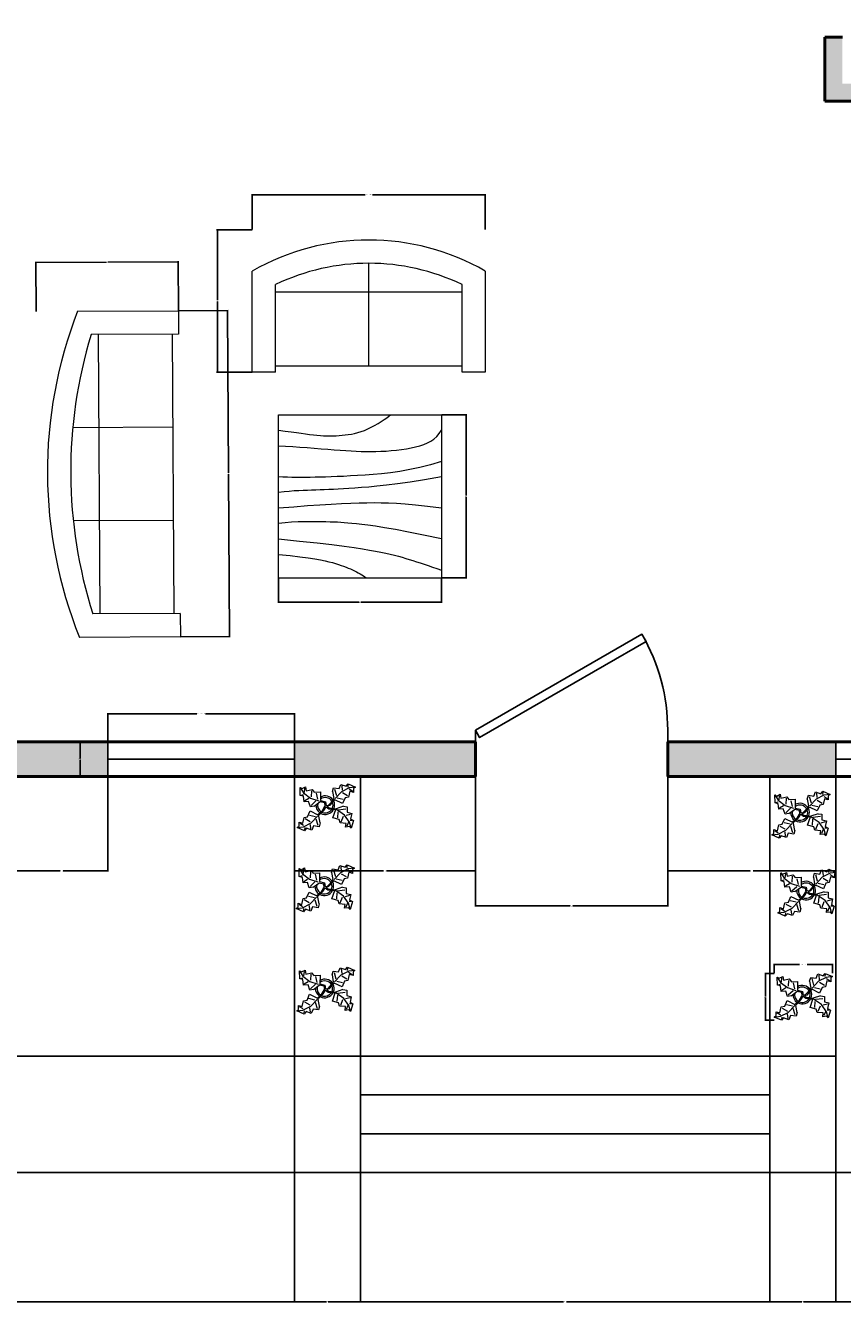
# Model space of a CAD drawing. Units: inches. Extents: x 4 to 671, y -79 to 570.
# Tile 2 of 7: x 198 to 408, y -79 to 250. Entities that reach past the tile are written whole.
import ezdxf

# ---------------------------------------------------------------- set-up
doc = ezdxf.new("R2010")
doc.units = ezdxf.units.IN
doc.header["$MEASUREMENT"] = 0
for name, color, linetype, lineweight in [('A-ANNO-DIMS', 2, 'Continuous', 18), ('A-FLOR-STRS', 7, 'Continuous', 25), ('A-WALL', 7, 'Continuous', 50), ('A-WALL-PATT', 251, 'Continuous', 13), ('doors', 40, 'Continuous', 25), ('furniture', 220, 'Continuous', 18), ('L-PLNT', 114, 'Continuous', 18), ('window', 30, 'Continuous', 25)]:
    doc.layers.add(name, color=color, linetype=linetype, lineweight=lineweight)
doc.styles.get("Standard").update_dxf_attribs({"font": 'arial.ttf'})
doc.dimstyles.get("Standard").update_dxf_attribs({"dimtxt": 0.18, "dimasz": 0.18, "dimexe": 0.18, "dimexo": 0.0625, "dimgap": 0.09, "dimtad": 0, "dimtih": 1, "dimtoh": 1, "dimdec": 4, "dimzin": 0, "dimdsep": 46, "dimtxsty": 'Standard', "dimcen": 0.09, "dimadec": 0, "dimazin": 0, "dimtfac": 1, "dimtdec": 4, "dimtofl": 0, "dimtmove": 0, "dimatfit": 3, "dimfxl": 1, "dimtolj": 1, "dimtzin": 0, "dimarcsym": 0})

# ---------------------------------------------------------------- blocks, each defined once
blk = doc.blocks.new('*U9')
for p, q in [((0, 0), (0, -6)), ((40, 0), (40, -6))]:
    blk.add_line(p, q)
blk.add_lwpolyline([(0, 0), (34.64, 20), (35.52, 18.48), (0.87, -1.52)], close=True)
blk.add_arc((0, 0), 40, 0, 30)
blk = doc.blocks.new('Sofa - Roundback 7 ft.')
for p, q in [((-12.00002, -32.4421), (-12.00003, -6.5971)), ((11.99997, -32.4421), (11.99998, -6.5971)), ((-36.000027, -34), (-36.000027, -11.4696)), ((35.99998, -34), (35.99998, -11.4696)), ((-35.999844, -13.3819), (35.9998, -13.3819)), ((-36.000027, -32.4421), (35.99998, -32.4421))]:
    blk.add_line(p, q)
for points in [[(-36.000027, -34), (-42.000027, -34), (-42.000027, -8)], [(41.99998, -8), (41.99998, -34), (35.99998, -34)]]:
    blk.add_lwpolyline(points)
for centre, radius, start, end in [((0, -114.25), 114.25, 68.43141, 111.5686), ((-0.00001, -127.1968), 121.1968, 72.72033, 107.2797)]:
    blk.add_arc(centre, radius, start, end)
blk = doc.blocks.new('Sofa - Roundback Loveseat 5 ft.')
for p, q in [((0, -32.44198), (0, -5.99998)), ((-24, -33.99998), (-24, -11.46958)), ((24.00004, -33.99998), (24.00004, -11.46958)), ((-23.9998, -13.38178), (23.99986, -13.38178)), ((-24, -32.44198), (24.00004, -32.44198))]:
    blk.add_line(p, q)
for points in [[(-24, -33.99998), (-30, -33.99998), (-30, -7.99998)], [(30.00004, -7.99998), (30.00004, -33.99998), (24.00004, -33.99998)]]:
    blk.add_lwpolyline(points)
for centre, radius, start, end in [((0, -60.24998), 60.24998, 60.13715, 119.8628), ((0, -61.38438), 55.38444, 64.32083, 115.6792)]:
    blk.add_arc(centre, radius, start, end)
blk = doc.blocks.new('Table - Square Woodgrain 42 x 42 in.')
blk.add_line((0, -42), (42, -42))
for points in [[(0, -4), (1.704, -4.2172), (3.2358, -4.4188), (4.615, -4.604), (5.8615, -4.7721), (6.9951, -4.9224), (8.0357, -5.0541), (9.0031, -5.1667), (9.9171, -5.2594), (10.7951, -5.3316), (11.6445, -5.3836), (12.4702, -5.4157), (13.277, -5.4283), (14.0698, -5.4217), (14.8535, -5.3964), (15.6331, -5.3526), (16.4133, -5.2908), (17.1986, -5.2103), (17.9913, -5.1062), (18.793, -4.9727), (19.6056, -4.8038), (20.4307, -4.5937), (21.2701, -4.3365), (22.1256, -4.0262), (22.9989, -3.6571), (23.888, -3.2272), (24.7756, -2.7516), (25.6408, -2.2491), (26.4624, -1.7387), (27.2195, -1.2395), (27.891, -0.7703), (28.456, -0.3501), (28.8934, 0.002)], [(0, -42), (0, 0), (42, 0), (42, -42)], [(0, -8), (1.8203, -8.1001), (3.6741, -8.2149), (5.5411, -8.3408), (7.4011, -8.4741), (9.2339, -8.6112), (11.0193, -8.7484), (12.7371, -8.8821), (14.3671, -9.0086), (15.8954, -9.1246), (17.3337, -9.2278), (18.6997, -9.3159), (20.0116, -9.387), (21.2871, -9.4389), (22.5442, -9.4696), (23.8008, -9.477), (25.0749, -9.459), (26.3791, -9.4137), (27.7049, -9.3403), (29.0383, -9.2382), (30.3655, -9.1068), (31.6728, -8.9455), (32.9461, -8.7535), (34.1717, -8.5304), (35.3358, -8.2756), (36.4268, -7.9863), (37.443, -7.6521), (38.3849, -7.2603), (39.253, -6.7986), (40.048, -6.2542), (40.7705, -5.6147), (41.421, -4.8674), (42, -4)], [(42, -12), (39.1784, -12.8621), (36.4519, -13.5654), (33.8246, -14.1294), (31.3004, -14.5731), (28.8832, -14.9161), (26.577, -15.1775), (24.3858, -15.3768), (22.3136, -15.5332), (20.3622, -15.6632), (18.5254, -15.7718), (16.7947, -15.8612), (15.1618, -15.9338), (13.6183, -15.9916), (12.1558, -16.0369), (10.7659, -16.0718), (9.4403, -16.0987), (8.1703, -16.1191), (6.9461, -16.1325), (5.7577, -16.1377), (4.595, -16.1335), (3.4479, -16.1188), (2.3064, -16.0924), (1.1604, -16.0532), (0, -16)], [(42, -16), (37.6529, -16.7365), (33.8802, -17.329), (30.6179, -17.7961), (27.8015, -18.1561), (25.3668, -18.4275), (23.2497, -18.6288), (21.3859, -18.7785), (19.7111, -18.8949), (18.1693, -18.9939), (16.7375, -19.0795), (15.401, -19.1534), (14.1449, -19.217), (12.9544, -19.2717), (11.8148, -19.3191), (10.7113, -19.3606), (9.6291, -19.3976), (8.5534, -19.4323), (7.47, -19.4689), (6.3643, -19.5122), (5.222, -19.5672), (4.0288, -19.6386), (2.7703, -19.7313), (1.4321, -19.8501), (0, -20)], [(0, -24), (3.9243, -23.6805), (7.4766, -23.4138), (10.6891, -23.1954), (13.5943, -23.0205), (16.2247, -22.8847), (18.6125, -22.7832), (20.7903, -22.7116), (22.7903, -22.6651), (24.6563, -22.642), (26.4764, -22.6507), (28.35, -22.7024), (30.3766, -22.8084), (32.6555, -22.98), (35.2861, -23.2283), (38.3678, -23.5645), (42, -24)], [(42, -32), (37.392, -31.017), (33.4585, -30.2231), (30.1291, -29.5949), (27.3334, -29.109), (25.0009, -28.742), (23.0612, -28.4707), (21.4439, -28.2716), (20.0786, -28.1215), (18.8998, -28.0002), (17.8609, -27.9014), (16.9206, -27.8219), (16.0371, -27.7588), (15.1691, -27.709), (14.2748, -27.6693), (13.3128, -27.6368), (12.2415, -27.6083), (11.0295, -27.5824), (9.6867, -27.5643), (8.233, -27.5608), (6.6884, -27.5787), (5.0728, -27.6248), (3.4062, -27.7058), (1.7086, -27.8286), (0, -28)], [(0, -32), (5.4026, -32.5358), (9.9494, -33.019), (13.7424, -33.4553), (16.8834, -33.8505), (19.4743, -34.2106), (21.6171, -34.5413), (23.4136, -34.8486), (24.9657, -35.1382), (26.3614, -35.4156), (27.6332, -35.6841), (28.7995, -35.9467), (29.8788, -36.2064), (30.8897, -36.4661), (31.8507, -36.7288), (32.7802, -36.9973), (33.6968, -37.2747), (34.6175, -37.5635), (35.5531, -37.8651), (36.5128, -38.1805), (37.506, -38.5108), (38.5421, -38.8568), (39.6302, -39.2197), (40.7797, -39.6004), (42, -40)], [(0, -36), (3.0098, -36.2857), (5.5354, -36.5643), (7.6368, -36.8359), (9.374, -37.1009), (10.807, -37.3597), (11.9957, -37.6126), (13.0002, -37.8599), (13.8804, -38.102), (14.6874, -38.3393), (15.4365, -38.5729), (16.1338, -38.8041), (16.7858, -39.0341), (17.3987, -39.264), (17.9787, -39.4952), (18.5322, -39.7288), (19.0655, -39.9662), (19.5832, -40.2081), (20.0842, -40.4544), (20.5657, -40.7046), (21.0249, -40.9581), (21.459, -41.2144), (21.8653, -41.4731), (22.2409, -41.7335), (22.5831, -41.9951)]]:
    blk.add_lwpolyline(points)
blk = doc.blocks.new('Plant - Rubber or Philodendron')
for p, q in [((-16.2005, 11.4774), (-13.9899, 8.1064)), ((-16.2005, 11.4774), (-14.8639, 10.7964)), ((-16.0159, 6.3329), (-16.2005, 11.4774)), ((-14.8639, 10.7964), (-12.6195, 11.8975)), ((-13.3174, 8.325), (-13.0735, 11.0065)), ((-12.6195, 11.8975), (-12.1909, 9.4345)), ((-12.1909, 9.4345), (-8.3829, 10.3)), ((-8.8369, 9.409), (-9.0894, 5.6095)), ((-8.3829, 10.3), (-7.0549, 8.501)), ((-7.0549, 8.501), (-3.0284, 8.6941)), ((-3.0284, 8.6941), (-3.0709, 3.1041)), ((4.6914, 8.8812), (5.3859, 11.2828)), ((4.6914, 8.8812), (5.5014, 4.4831)), ((5.3859, 11.2828), (8.8871, 10.7908)), ((5.9878, 10.4842), (7.1971, 6.3869)), ((10.3916, 8.7942), (6.2847, 4.4028)), ((8.8871, 10.7908), (9.9809, 13.4933)), ((9.9809, 13.4933), (13.3837, 12.301)), ((15.3859, 11.3055), (10.3916, 8.7942)), ((10.5828, 12.6946), (10.8893, 9.7953)), ((13.3837, 12.301), (14.68, 13.9039)), ((14.5816, 13.2037), (14.3848, 11.8033)), ((14.68, 13.9039), (19.3848, 11.8146)), ((15.7909, 9.1065), (14.8995, 5.3044)), ((15.2875, 10.6053), (17.5907, 9.2105)), ((19.3848, 11.8146), (15.3859, 11.3055)), ((18.1925, 8.4119), (15.7909, 9.1065)), ((19.3848, 11.8146), (18.1868, 10.9119)), ((18.1868, 10.9119), (18.1925, 8.4119)), ((-14.0069, 5.8704), (-16.0159, 6.3329)), ((-15.3434, 6.5514), (-13.9984, 6.9884)), ((-13.5868, 2.2894), (-14.0069, 5.8704)), ((-13.9899, 8.1064), (-9.5434, 4.7185)), ((-10.6784, 2.491), (-13.5868, 2.2894)), ((-13.1329, 3.1804), (-10.6614, 4.727)), ((-9.5858, -0.8715), (-10.6784, 2.491)), ((-9.5434, 4.7185), (-4.1917, 2.9888)), ((-9.1318, 0.0195), (-5.9793, 2.9025)), ((-7.1228, -0.443), (-3.5248, 2.2131)), ((-4.8529, 4.012), (-5.7184, 7.82)), ((-3.5248, 2.2131), (-3.3011, 2.4355)), ((-3.3011, 2.4355), (-0.5306, 1.7947)), ((-3.0709, 3.1041), (0.0797, 2.3163)), ((-0.5306, 1.7947), (-0.2255, -0.5527)), ((-0.5306, 1.7947), (-0.5306, 1.7947)), ((0.0797, 2.3163), (0.4866, -0.031)), ((0.4866, -0.031), (2.1141, 0.2298)), ((2.1141, 0.2298), (5.4346, 3.9146)), ((6.1032, 3.6844), (2.8262, -0.031)), ((5.4346, 3.9146), (5.5014, 4.4831)), ((11.1089, 1.1958), (6.1032, 3.6844)), ((7.7005, 4.8881), (11.5025, 3.9967)), ((14.2977, 6.1031), (10.9934, 7.9956)), ((12.7005, 4.8994), (11.1089, 1.1958)), ((14.8995, 5.3044), (12.7005, 4.8994)), ((-14.4141, -11.4699), (-13.5228, -7.6679)), ((-13.5228, -7.6679), (-11.3237, -7.2629)), ((-11.3237, -7.2629), (-9.7321, -3.5593)), ((-6.3237, -7.2516), (-10.1257, -6.3602)), ((-9.7321, -3.5593), (-4.7264, -6.0479)), ((-7.1228, -0.443), (-9.5858, -0.8715)), ((-9.0148, -11.1577), (-4.9047, -6.8122)), ((-2.019, -3.6148), (-4.7264, -6.0479)), ((-4.1246, -6.8466), (-4.0579, -6.2781)), ((-3.3146, -11.2447), (-4.1246, -6.8466)), ((-4.0579, -6.2781), (-0.9375, -3.1608)), ((-2.019, -3.6148), (-0.2255, -0.5527)), ((-0.9375, -3.1608), (0.5883, -0.8135)), ((0.5883, -0.8135), (2.2447, -2.0916)), ((2.8262, -0.031), (1.3003, -0.5527)), ((1.3003, -0.5527), (2.4193, -1.4655)), ((2.2447, -2.0916), (6.7108, -2.6626)), ((2.4193, -1.4655), (6.895, -2.1175)), ((4.943, -7.9659), (6.7108, -2.6626)), ((8.8321, -9.0266), (4.943, -7.9659)), ((11.6605, -0.5413), (6.895, -2.1175)), ((12.3677, -6.1981), (7.219, -2.6772)), ((8.125, -4.0768), (7.7715, -7.9659)), ((8.3544, -2.7453), (13.1973, -2.1704)), ((10.2463, -10.4408), (11.6605, -6.9053)), ((11.6605, -0.5413), (14.1354, -0.8948)), ((15.5496, -10.7943), (12.3677, -6.1981)), ((16.2567, -5.8446), (13.4283, -6.5517)), ((14.1354, -0.8948), (14.1354, -4.4304)), ((14.1354, -4.4304), (16.9638, -5.1375)), ((16.9638, -5.1375), (16.2567, -8.673)), ((-18.008, -14.1781), (-16.8101, -13.2754)), ((-18.008, -14.1781), (-14.0091, -13.669)), ((-13.3032, -16.2674), (-18.008, -14.1781)), ((-16.8157, -10.7754), (-14.4141, -11.4699)), ((-16.8101, -13.2754), (-16.8157, -10.7754)), ((-13.9107, -12.9688), (-16.2139, -11.574)), ((-14.0091, -13.669), (-9.0148, -11.1577)), ((-12.0069, -14.6645), (-13.3032, -16.2674)), ((-13.2048, -15.5672), (-13.008, -14.1668)), ((-12.921, -8.4665), (-9.6166, -10.359)), ((-8.6042, -15.8568), (-12.0069, -14.6645)), ((-9.206, -15.0581), (-9.5126, -12.1588)), ((-7.5103, -13.1543), (-8.6042, -15.8568)), ((-4.0092, -13.6463), (-7.5103, -13.1543)), ((-4.611, -12.8477), (-5.8203, -8.7504)), ((-3.3146, -11.2447), (-4.0092, -13.6463)), ((9.5392, -11.1479), (8.8321, -9.0266)), ((13.4283, -11.5015), (9.5392, -11.1479)), ((13.0748, -13.9763), (13.4283, -11.5015)), ((15.5496, -13.6228), (13.0748, -13.9763)), ((14.8425, -10.7943), (13.7819, -13.2692)), ((16.6103, -14.6834), (15.5496, -10.7943)), ((16.6103, -14.6834), (15.5496, -13.6228)), ((17.3174, -9.7337), (15.9032, -9.7337)), ((16.2567, -8.673), (18.0245, -9.7337)), ((18.0245, -9.7337), (16.6103, -14.6834))]:
    blk.add_line(p, q)
for centre, radius, start, end in [((0.0308, 0.1664), 6, 178.6147, 235.1169), ((0.0308, 0.1664), 5, 168.1647, 238.6725), ((0, 0), 6.1275, 34.37569, 120.1028), ((-0.0601, -0.2075), 5.2461, 33.82192, 124.9414), ((-0.2664, 0.1682), 5.2775, 338.4094, 20.03007), ((-0.098, 0.1364), 6.1288, 341.2017, 26.09184), ((-0.0234, 0.3825), 6.1492, 242.5812, 331.2714), ((-0.1102, 0.4886), 5.2883, 247.3711, 327.472)]:
    blk.add_arc(centre, radius, start, end)
blk = doc.blocks.new('WIN-48')
for p, q in [((0, 9), (0, 0)), ((48, 9), (0, 9)), ((0, 9), (0, 4.5)), ((48, 0), (48, 9)), ((0, 4.5), (48, 4.5)), ((0, 0), (48, 0))]:
    blk.add_line(p, q)
blk = doc.blocks.new('*D25')
at = {"layer": 'A-ANNO-DIMS', "color": 0, "lineweight": -2, "transparency": 16777216}
for p, q in [((218.8, 65.41), (218.8, 72.73)), ((218.98, 72.55), (241.68, 72.55)), ((266.62, 72.55), (243.92, 72.55)), ((266.8, 65.41), (266.8, 72.73))]:
    blk.add_line(p, q, dxfattribs=at)
at = {"layer": 'A-ANNO-DIMS', "color": 0, "transparency": 16777216}
for points in [[(218.98, 72.58), (218.98, 72.52), (218.8, 72.55)], [(266.62, 72.58), (266.62, 72.52), (266.8, 72.55)]]:
    blk.add_solid(points, dxfattribs=at)
at = {"layer": 'Defpoints', "color": 0, "transparency": 16777216}
for p in [(266.8, 72.55), (218.8, 65.35), (266.8, 65.35)]:
    blk.add_point(p, dxfattribs=at)
at = {"layer": 'A-ANNO-DIMS', "color": 0, "transparency": 16777216, "insert": (242.8, 72.55), "char_height": 0.18, "attachment_point": 5}
blk.add_mtext('\\A1;WINDOW 48 TYP.', dxfattribs=at)
blk = doc.blocks.new('*D26')
at = {"layer": 'A-ANNO-DIMS', "color": 0, "lineweight": -2, "transparency": 16777216}
for p, q in [((218.74, 65.35), (211.42, 65.35)), ((211.6, 65.17), (211.6, 61.03)), ((211.6, 56.53), (211.6, 60.67)), ((218.74, 56.35), (211.42, 56.35))]:
    blk.add_line(p, q, dxfattribs=at)
at = {"layer": 'A-ANNO-DIMS', "color": 0, "transparency": 16777216}
for points in [[(211.57, 65.17), (211.63, 65.17), (211.6, 65.35)], [(211.57, 56.53), (211.63, 56.53), (211.6, 56.35)]]:
    blk.add_solid(points, dxfattribs=at)
at = {"layer": 'Defpoints', "color": 0, "transparency": 16777216}
for p in [(211.6, 65.35), (218.8, 65.35), (218.8, 56.35)]:
    blk.add_point(p, dxfattribs=at)
at = {"layer": 'A-ANNO-DIMS', "color": 0, "transparency": 16777216, "insert": (211.6, 60.85), "char_height": 0.18, "attachment_point": 5}
blk.add_mtext('\\A1;9 TYP.', dxfattribs=at)
blk = doc.blocks.new('*D37')
at = {"layer": 'A-ANNO-DIMS', "color": 0, "lineweight": -2, "transparency": 16777216}
for p, q in [((237.02, 176.38), (249.74, 176.46)), ((249.56, 176.28), (249.81, 134.64)), ((250.06, 92.64), (249.81, 134.27)), ((237.52, 92.38), (250.24, 92.46))]:
    blk.add_line(p, q, dxfattribs=at)
at = {"layer": 'A-ANNO-DIMS', "color": 0, "transparency": 16777216}
for points in [[(249.59, 176.28), (249.53, 176.28), (249.56, 176.46)], [(250.09, 92.64), (250.03, 92.64), (250.06, 92.46)]]:
    blk.add_solid(points, dxfattribs=at)
at = {"layer": 'Defpoints', "color": 0, "transparency": 16777216}
for p in [(236.96, 176.38), (249.56, 176.46), (237.46, 92.38)]:
    blk.add_point(p, dxfattribs=at)
at = {"layer": 'A-ANNO-DIMS', "color": 0, "transparency": 16777216, "insert": (249.81, 134.46), "char_height": 0.18, "attachment_point": 5}
blk.add_mtext('\\A1;SOFA 84', dxfattribs=at)
blk = doc.blocks.new('*D38')
at = {"layer": 'A-ANNO-DIMS', "color": 0, "lineweight": -2, "transparency": 16777216}
for p, q in [((200.29, 176.22), (200.21, 188.94)), ((200.39, 188.76), (218.33, 188.87)), ((236.7, 188.98), (218.77, 188.87)), ((236.96, 176.44), (236.88, 189.16))]:
    blk.add_line(p, q, dxfattribs=at)
at = {"layer": 'A-ANNO-DIMS', "color": 0, "transparency": 16777216}
for points in [[(200.39, 188.79), (200.39, 188.73), (200.21, 188.76)], [(236.7, 189.01), (236.7, 188.95), (236.88, 188.98)]]:
    blk.add_solid(points, dxfattribs=at)
at = {"layer": 'Defpoints', "color": 0, "transparency": 16777216}
for p in [(200.21, 188.76), (200.29, 176.16), (236.96, 176.38)]:
    blk.add_point(p, dxfattribs=at)
at = {"layer": 'A-ANNO-DIMS', "color": 0, "transparency": 16777216, "insert": (218.55, 188.87), "char_height": 0.18, "attachment_point": 5}
blk.add_mtext('\\A1;37', dxfattribs=at)
blk = doc.blocks.new('*D39')
at = {"layer": 'A-ANNO-DIMS', "color": 0, "lineweight": -2, "transparency": 16777216}
for p, q in [((255.97, 197.32), (255.97, 206.44)), ((256.15, 206.26), (285.06, 206.26)), ((315.79, 206.26), (286.89, 206.26)), ((315.97, 197.32), (315.97, 206.44))]:
    blk.add_line(p, q, dxfattribs=at)
at = {"layer": 'A-ANNO-DIMS', "color": 0, "transparency": 16777216}
for points in [[(256.15, 206.29), (256.15, 206.23), (255.97, 206.26)], [(315.79, 206.29), (315.79, 206.23), (315.97, 206.26)]]:
    blk.add_solid(points, dxfattribs=at)
at = {"layer": 'Defpoints', "color": 0, "transparency": 16777216}
for p in [(315.97, 206.26), (255.97, 197.26), (315.97, 197.26)]:
    blk.add_point(p, dxfattribs=at)
at = {"layer": 'A-ANNO-DIMS', "color": 0, "transparency": 16777216, "insert": (285.97, 206.26), "char_height": 0.18, "attachment_point": 5}
blk.add_mtext('\\A1;LOVESEAT 60', dxfattribs=at)
blk = doc.blocks.new('*D40')
at = {"layer": 'A-ANNO-DIMS', "color": 0, "lineweight": -2, "transparency": 16777216}
for p, q in [((255.91, 197.26), (246.79, 197.26)), ((246.97, 197.08), (246.97, 179.1)), ((246.97, 160.77), (246.97, 178.74)), ((255.91, 160.59), (246.79, 160.59))]:
    blk.add_line(p, q, dxfattribs=at)
at = {"layer": 'A-ANNO-DIMS', "color": 0, "transparency": 16777216}
for points in [[(246.94, 197.08), (247, 197.08), (246.97, 197.26)], [(246.94, 160.77), (247, 160.77), (246.97, 160.59)]]:
    blk.add_solid(points, dxfattribs=at)
at = {"layer": 'Defpoints', "color": 0, "transparency": 16777216}
for p in [(246.97, 197.26), (255.97, 197.26), (255.97, 160.59)]:
    blk.add_point(p, dxfattribs=at)
at = {"layer": 'A-ANNO-DIMS', "color": 0, "transparency": 16777216, "insert": (246.97, 178.92), "char_height": 0.18, "attachment_point": 5}
blk.add_mtext('\\A1;37', dxfattribs=at)
blk = doc.blocks.new('*D43')
at = {"layer": 'A-ANNO-DIMS', "color": 0, "lineweight": -2, "transparency": 16777216}
for p, q in [((304.76, 149.57), (311.18, 149.57)), ((311, 149.39), (311, 128.75)), ((311, 107.75), (311, 128.39)), ((304.76, 107.57), (311.18, 107.57))]:
    blk.add_line(p, q, dxfattribs=at)
at = {"layer": 'A-ANNO-DIMS', "color": 0, "transparency": 16777216}
for points in [[(310.97, 149.39), (311.03, 149.39), (311, 149.57)], [(310.97, 107.75), (311.03, 107.75), (311, 107.57)]]:
    blk.add_solid(points, dxfattribs=at)
at = {"layer": 'Defpoints', "color": 0, "transparency": 16777216}
for p in [(304.7, 149.57), (311, 149.57), (304.7, 107.57)]:
    blk.add_point(p, dxfattribs=at)
at = {"layer": 'A-ANNO-DIMS', "color": 0, "transparency": 16777216, "insert": (311, 128.57), "char_height": 0.18, "attachment_point": 5}
blk.add_mtext('\\A1;TABLE 42', dxfattribs=at)
blk = doc.blocks.new('*D44')
at = {"layer": 'A-ANNO-DIMS', "color": 0, "lineweight": -2, "transparency": 16777216}
for p, q in [((262.7, 107.51), (262.7, 101.09)), ((304.7, 107.51), (304.7, 101.09)), ((262.88, 101.27), (283.48, 101.27)), ((304.52, 101.27), (283.92, 101.27))]:
    blk.add_line(p, q, dxfattribs=at)
at = {"layer": 'A-ANNO-DIMS', "color": 0, "transparency": 16777216}
for points in [[(262.88, 101.3), (262.88, 101.24), (262.7, 101.27)], [(304.52, 101.3), (304.52, 101.24), (304.7, 101.27)]]:
    blk.add_solid(points, dxfattribs=at)
at = {"layer": 'Defpoints', "color": 0, "transparency": 16777216}
for p in [(262.7, 107.57), (304.7, 107.57), (304.7, 101.27)]:
    blk.add_point(p, dxfattribs=at)
at = {"layer": 'A-ANNO-DIMS', "color": 0, "transparency": 16777216, "insert": (283.7, 101.27), "char_height": 0.18, "attachment_point": 5}
blk.add_mtext('\\A1;42', dxfattribs=at)
blk = doc.blocks.new('*D47')
at = {"layer": 'A-ANNO-DIMS', "color": 0, "lineweight": -2, "transparency": 16777216}
for p, q in [((390.39, 5.73), (390.39, 8.09)), ((390.57, 7.91), (396.92, 7.91)), ((405.21, 7.91), (398.85, 7.91)), ((405.39, 5.73), (405.39, 8.09))]:
    blk.add_line(p, q, dxfattribs=at)
at = {"layer": 'A-ANNO-DIMS', "color": 0, "transparency": 16777216}
for points in [[(390.57, 7.94), (390.57, 7.88), (390.39, 7.91)], [(405.21, 7.94), (405.21, 7.88), (405.39, 7.91)]]:
    blk.add_solid(points, dxfattribs=at)
at = {"layer": 'Defpoints', "color": 0, "transparency": 16777216}
for p in [(405.39, 7.91), (390.39, 5.66), (405.39, 5.66)]:
    blk.add_point(p, dxfattribs=at)
at = {"layer": 'A-ANNO-DIMS', "color": 0, "transparency": 16777216, "insert": (397.89, 7.91), "char_height": 0.18, "attachment_point": 5}
blk.add_mtext('\\A1;PLANT 15 TYP.', dxfattribs=at)
blk = doc.blocks.new('*D48')
at = {"layer": 'A-ANNO-DIMS', "color": 0, "lineweight": -2, "transparency": 16777216}
for p, q in [((390.33, 5.66), (387.96, 5.66)), ((388.14, 5.48), (388.14, -0.21)), ((388.14, -6.26), (388.14, -0.57)), ((390.33, -6.44), (387.96, -6.44))]:
    blk.add_line(p, q, dxfattribs=at)
at = {"layer": 'A-ANNO-DIMS', "color": 0, "transparency": 16777216}
for points in [[(388.11, 5.48), (388.17, 5.48), (388.14, 5.66)], [(388.11, -6.26), (388.17, -6.26), (388.14, -6.44)]]:
    blk.add_solid(points, dxfattribs=at)
at = {"layer": 'Defpoints', "color": 0, "transparency": 16777216}
for p in [(388.14, 5.66), (390.39, 5.66), (390.39, -6.44)]:
    blk.add_point(p, dxfattribs=at)
at = {"layer": 'A-ANNO-DIMS', "color": 0, "transparency": 16777216, "insert": (388.14, -0.39), "char_height": 0.18, "attachment_point": 5}
blk.add_mtext('\\A1;12 TYP.', dxfattribs=at)
blk = doc.blocks.new('*D50')
at = {"layer": 'A-ANNO-DIMS', "color": 0, "lineweight": -2, "transparency": 16777216}
for p, q in [((637.5, 536.35), (670.92, 536.35)), ((670.74, 536.17), (670.74, 245.53)), ((670.74, -45.47), (670.74, 245.17)), ((389.27, -45.65), (670.92, -45.65))]:
    blk.add_line(p, q, dxfattribs=at)
at = {"layer": 'A-ANNO-DIMS', "color": 0, "transparency": 16777216}
for points in [[(670.71, 536.17), (670.77, 536.17), (670.74, 536.35)], [(670.71, -45.47), (670.77, -45.47), (670.74, -45.65)]]:
    blk.add_solid(points, dxfattribs=at)
at = {"layer": 'Defpoints', "color": 0, "transparency": 16777216}
for p in [(637.44, 536.35), (389.21, -45.65), (670.74, -45.65)]:
    blk.add_point(p, dxfattribs=at)
at = {"layer": 'A-ANNO-DIMS', "color": 0, "transparency": 16777216, "insert": (670.74, 245.35), "char_height": 0.18, "attachment_point": 5}
blk.add_mtext('\\A1;582', dxfattribs=at)
blk = doc.blocks.new('*D52')
at = {"layer": 'A-ANNO-DIMS', "color": 0, "lineweight": -2, "transparency": 16777216}
for p, q in [((37.38, 56.35), (3.96, 56.35)), ((4.14, 56.17), (4.14, 20.53)), ((4.14, -15.47), (4.14, 20.17)), ((266.74, -15.65), (3.96, -15.65))]:
    blk.add_line(p, q, dxfattribs=at)
at = {"layer": 'A-ANNO-DIMS', "color": 0, "transparency": 16777216}
for points in [[(4.11, 56.17), (4.17, 56.17), (4.14, 56.35)], [(4.11, -15.47), (4.17, -15.47), (4.14, -15.65)]]:
    blk.add_solid(points, dxfattribs=at)
at = {"layer": 'Defpoints', "color": 0, "transparency": 16777216}
for p in [(4.14, 56.35), (37.44, 56.35), (266.8, -15.65)]:
    blk.add_point(p, dxfattribs=at)
at = {"layer": 'A-ANNO-DIMS', "color": 0, "transparency": 16777216, "insert": (4.14, 20.35), "char_height": 0.18, "attachment_point": 5}
blk.add_mtext('\\A1;72', dxfattribs=at)
blk = doc.blocks.new('*D53')
at = {"layer": 'A-ANNO-DIMS', "color": 0, "lineweight": -2, "transparency": 16777216}
for p, q in [((266.74, -15.65), (3.96, -15.65)), ((4.14, -15.83), (4.14, -30.47)), ((4.14, -45.47), (4.14, -30.83)), ((283.74, -45.65), (3.96, -45.65))]:
    blk.add_line(p, q, dxfattribs=at)
at = {"layer": 'A-ANNO-DIMS', "color": 0, "transparency": 16777216}
for points in [[(4.11, -15.83), (4.17, -15.83), (4.14, -15.65)], [(4.11, -45.47), (4.17, -45.47), (4.14, -45.65)]]:
    blk.add_solid(points, dxfattribs=at)
at = {"layer": 'Defpoints', "color": 0, "transparency": 16777216}
for p in [(4.14, -15.65), (266.8, -15.65), (283.8, -45.65)]:
    blk.add_point(p, dxfattribs=at)
at = {"layer": 'A-ANNO-DIMS', "color": 0, "transparency": 16777216, "insert": (4.14, -30.65), "char_height": 0.18, "attachment_point": 5}
blk.add_mtext('\\A1;30', dxfattribs=at)
blk = doc.blocks.new('*D54')
at = {"layer": 'A-ANNO-DIMS', "color": 0, "lineweight": -2, "transparency": 16777216}
for p, q in [((37.44, 56.29), (37.44, -79.13)), ((266.8, -15.71), (266.8, -79.13)), ((37.62, -78.95), (151.65, -78.95)), ((266.62, -78.95), (152.59, -78.95))]:
    blk.add_line(p, q, dxfattribs=at)
at = {"layer": 'A-ANNO-DIMS', "color": 0, "transparency": 16777216}
for points in [[(37.62, -78.92), (37.62, -78.98), (37.44, -78.95)], [(266.62, -78.92), (266.62, -78.98), (266.8, -78.95)]]:
    blk.add_solid(points, dxfattribs=at)
at = {"layer": 'Defpoints', "color": 0, "transparency": 16777216}
for p in [(37.44, 56.35), (266.8, -15.65), (266.8, -78.95)]:
    blk.add_point(p, dxfattribs=at)
at = {"layer": 'A-ANNO-DIMS', "color": 0, "transparency": 16777216, "insert": (152.12, -78.95), "char_height": 0.18, "attachment_point": 5}
blk.add_mtext('\\A1;229.36', dxfattribs=at)
blk = doc.blocks.new('*D55')
at = {"layer": 'A-ANNO-DIMS', "color": 0, "lineweight": -2, "transparency": 16777216}
for p, q in [((266.8, -15.71), (266.8, -79.13)), ((283.8, -15.71), (283.8, -79.13)), ((266.98, -78.95), (275.09, -78.95)), ((283.62, -78.95), (275.51, -78.95))]:
    blk.add_line(p, q, dxfattribs=at)
at = {"layer": 'A-ANNO-DIMS', "color": 0, "transparency": 16777216}
for points in [[(266.98, -78.92), (266.98, -78.98), (266.8, -78.95)], [(283.62, -78.92), (283.62, -78.98), (283.8, -78.95)]]:
    blk.add_solid(points, dxfattribs=at)
at = {"layer": 'Defpoints', "color": 0, "transparency": 16777216}
for p in [(266.8, -15.65), (283.8, -15.65), (283.8, -78.95)]:
    blk.add_point(p, dxfattribs=at)
at = {"layer": 'A-ANNO-DIMS', "color": 0, "transparency": 16777216, "insert": (275.3, -78.95), "char_height": 0.18, "attachment_point": 5}
blk.add_mtext('\\A1;17', dxfattribs=at)
blk = doc.blocks.new('*D56')
at = {"layer": 'A-ANNO-DIMS', "color": 0, "lineweight": -2, "transparency": 16777216}
for p, q in [((283.8, -45.71), (283.8, -79.13)), ((389.21, -45.71), (389.21, -79.13)), ((283.98, -78.95), (336.12, -78.95)), ((389.03, -78.95), (336.89, -78.95))]:
    blk.add_line(p, q, dxfattribs=at)
at = {"layer": 'A-ANNO-DIMS', "color": 0, "transparency": 16777216}
for points in [[(283.98, -78.92), (283.98, -78.98), (283.8, -78.95)], [(389.03, -78.92), (389.03, -78.98), (389.21, -78.95)]]:
    blk.add_solid(points, dxfattribs=at)
at = {"layer": 'Defpoints', "color": 0, "transparency": 16777216}
for p in [(283.8, -45.65), (389.21, -45.65), (389.21, -78.95)]:
    blk.add_point(p, dxfattribs=at)
at = {"layer": 'A-ANNO-DIMS', "color": 0, "transparency": 16777216, "insert": (336.5, -78.95), "char_height": 0.18, "attachment_point": 5}
blk.add_mtext('\\A1;105.4', dxfattribs=at)
blk = doc.blocks.new('*D57')
at = {"layer": 'A-ANNO-DIMS', "color": 0, "lineweight": -2, "transparency": 16777216}
for p, q in [((389.21, -15.71), (389.21, -79.13)), ((406.21, -15.71), (406.21, -79.13)), ((389.39, -78.95), (397.5, -78.95)), ((406.03, -78.95), (397.92, -78.95))]:
    blk.add_line(p, q, dxfattribs=at)
at = {"layer": 'A-ANNO-DIMS', "color": 0, "transparency": 16777216}
for points in [[(389.39, -78.92), (389.39, -78.98), (389.21, -78.95)], [(406.03, -78.92), (406.03, -78.98), (406.21, -78.95)]]:
    blk.add_solid(points, dxfattribs=at)
at = {"layer": 'Defpoints', "color": 0, "transparency": 16777216}
for p in [(389.21, -15.65), (406.21, -15.65), (406.21, -78.95)]:
    blk.add_point(p, dxfattribs=at)
at = {"layer": 'A-ANNO-DIMS', "color": 0, "transparency": 16777216, "insert": (397.71, -78.95), "char_height": 0.18, "attachment_point": 5}
blk.add_mtext('\\A1;17', dxfattribs=at)
blk = doc.blocks.new('*D58')
at = {"layer": 'A-ANNO-DIMS', "color": 0, "lineweight": -2, "transparency": 16777216}
for p, q in [((637.44, 56.29), (637.44, -79.13)), ((406.21, -15.71), (406.21, -79.13)), ((406.39, -78.95), (521.36, -78.95)), ((637.26, -78.95), (522.29, -78.95))]:
    blk.add_line(p, q, dxfattribs=at)
at = {"layer": 'A-ANNO-DIMS', "color": 0, "transparency": 16777216}
for points in [[(406.39, -78.92), (406.39, -78.98), (406.21, -78.95)], [(637.26, -78.92), (637.26, -78.98), (637.44, -78.95)]]:
    blk.add_solid(points, dxfattribs=at)
at = {"layer": 'Defpoints', "color": 0, "transparency": 16777216}
for p in [(637.44, 56.35), (406.21, -15.65), (637.44, -78.95)]:
    blk.add_point(p, dxfattribs=at)
at = {"layer": 'A-ANNO-DIMS', "color": 0, "transparency": 16777216, "insert": (521.82, -78.95), "char_height": 0.18, "attachment_point": 5}
blk.add_mtext('\\A1;231.23', dxfattribs=at)
blk = doc.blocks.new('*D61')
at = {"layer": 'A-ANNO-DIMS', "color": 0, "lineweight": -2, "transparency": 16777216}
for p, q in [((313.44, 56.29), (313.44, 22.87)), ((362.94, 56.29), (362.94, 22.87)), ((313.62, 23.05), (337.86, 23.05)), ((362.76, 23.05), (338.52, 23.05))]:
    blk.add_line(p, q, dxfattribs=at)
at = {"layer": 'A-ANNO-DIMS', "color": 0, "transparency": 16777216}
for points in [[(313.62, 23.08), (313.62, 23.02), (313.44, 23.05)], [(362.76, 23.08), (362.76, 23.02), (362.94, 23.05)]]:
    blk.add_solid(points, dxfattribs=at)
at = {"layer": 'Defpoints', "color": 0, "transparency": 16777216}
for p in [(313.44, 56.35), (362.94, 56.35), (313.44, 23.05)]:
    blk.add_point(p, dxfattribs=at)
at = {"layer": 'A-ANNO-DIMS', "color": 0, "transparency": 16777216, "insert": (338.19, 23.05), "char_height": 0.18, "attachment_point": 5}
blk.add_mtext('\\A1;49.5', dxfattribs=at)
blk = doc.blocks.new('*D85')
at = {"layer": 'A-ANNO-DIMS', "color": 0, "lineweight": -2, "transparency": 16777216}
for p, q in [((194.94, 65.29), (194.94, 31.87)), ((218.8, 65.29), (218.8, 31.87)), ((195.12, 32.05), (206.47, 32.05)), ((218.62, 32.05), (207.27, 32.05))]:
    blk.add_line(p, q, dxfattribs=at)
at = {"layer": 'A-ANNO-DIMS', "color": 0, "transparency": 16777216}
for points in [[(195.12, 32.08), (195.12, 32.02), (194.94, 32.05)], [(218.62, 32.08), (218.62, 32.02), (218.8, 32.05)]]:
    blk.add_solid(points, dxfattribs=at)
at = {"layer": 'Defpoints', "color": 0, "transparency": 16777216}
for p in [(194.94, 65.35), (218.8, 65.35), (194.94, 32.05)]:
    blk.add_point(p, dxfattribs=at)
at = {"layer": 'A-ANNO-DIMS', "color": 0, "transparency": 16777216, "insert": (206.87, 32.05), "char_height": 0.18, "attachment_point": 5}
blk.add_mtext('\\A1;23.86', dxfattribs=at)
blk = doc.blocks.new('*D86')
at = {"layer": 'A-ANNO-DIMS', "color": 0, "lineweight": -2, "transparency": 16777216}
for p, q in [((266.8, 65.29), (266.8, 31.87)), ((313.44, 65.29), (313.44, 31.87)), ((266.98, 32.05), (289.72, 32.05)), ((313.26, 32.05), (290.52, 32.05))]:
    blk.add_line(p, q, dxfattribs=at)
at = {"layer": 'A-ANNO-DIMS', "color": 0, "transparency": 16777216}
for points in [[(266.98, 32.08), (266.98, 32.02), (266.8, 32.05)], [(313.26, 32.08), (313.26, 32.02), (313.44, 32.05)]]:
    blk.add_solid(points, dxfattribs=at)
at = {"layer": 'Defpoints', "color": 0, "transparency": 16777216}
for p in [(266.8, 65.35), (313.44, 65.35), (266.8, 32.05)]:
    blk.add_point(p, dxfattribs=at)
at = {"layer": 'A-ANNO-DIMS', "color": 0, "transparency": 16777216, "insert": (290.12, 32.05), "char_height": 0.18, "attachment_point": 5}
blk.add_mtext('\\A1;46.64', dxfattribs=at)
blk = doc.blocks.new('*D87')
at = {"layer": 'A-ANNO-DIMS', "color": 0, "lineweight": -2, "transparency": 16777216}
for p, q in [((362.94, 65.29), (362.94, 31.87)), ((406.21, 65.29), (406.21, 31.87)), ((363.12, 32.05), (384.18, 32.05)), ((406.03, 32.05), (384.97, 32.05))]:
    blk.add_line(p, q, dxfattribs=at)
at = {"layer": 'A-ANNO-DIMS', "color": 0, "transparency": 16777216}
for points in [[(363.12, 32.08), (363.12, 32.02), (362.94, 32.05)], [(406.03, 32.08), (406.03, 32.02), (406.21, 32.05)]]:
    blk.add_solid(points, dxfattribs=at)
at = {"layer": 'Defpoints', "color": 0, "transparency": 16777216}
for p in [(362.94, 65.35), (406.21, 65.35), (362.94, 32.05)]:
    blk.add_point(p, dxfattribs=at)
at = {"layer": 'A-ANNO-DIMS', "color": 0, "transparency": 16777216, "insert": (384.57, 32.05), "char_height": 0.18, "attachment_point": 5}
blk.add_mtext('\\A1;43.27', dxfattribs=at)

msp = doc.modelspace()

# ---------------------------------------------------------------- hatches: boundary and pattern name
at = {"layer": 'A-WALL-PATT'}
h = msp.add_hatch(color=256, dxfattribs=at)
h.dxf.hatch_style = 1
h.paths.add_polyline_path([(46.4392, 165.2664), (37.4392, 165.2664), (37.4392, 108.5522), (41.9392, 108.5522), (46.4392, 108.5522), (46.4392, 117.8513), (151.434, 117.8513), (151.434, 120.1013), (151.434, 122.3513), (46.4392, 122.3513)], flags=17)
h.paths.add_polyline_path([(194.9392, 203.3513), (190.4392, 203.3513), (190.4392, 122.3513), (187.434, 122.3513), (187.434, 117.8513), (190.4392, 117.8513), (190.4392, 65.3513), (46.4392, 65.3513), (46.4392, 72.5522), (37.4392, 72.5522), (37.4392, 56.3513), (218.8007, 56.3513), (218.8007, 65.3513), (194.9392, 65.3513)])
h.paths.add_polyline_path([(46.4392, 242.3513), (190.4392, 242.3513), (190.4392, 239.3513), (194.9392, 239.3513), (194.9392, 249.8513), (190.4392, 249.8513), (190.4392, 246.8513), (46.4392, 246.8513), (46.4392, 303.5372), (37.4392, 303.5372), (37.4392, 201.2664), (41.9392, 201.2664), (46.4392, 201.2664)])
h.paths.add_polyline_path([(46.4392, 378.8513), (190.4392, 378.8513), (190.4392, 285.8513), (194.9392, 285.8513), (194.9392, 378.8513), (295.4392, 378.8513), (295.4392, 386.3513), (290.9392, 386.3513), (290.9392, 383.3513), (122.9392, 383.3513), (122.9392, 386.3513), (118.4392, 386.3513), (118.4392, 383.3513), (46.4392, 383.3513), (46.4392, 438.8513), (79.4392, 438.8513), (79.4392, 443.3513), (46.4392, 443.3513), (46.4392, 527.3513), (57.0095, 527.3513), (57.0095, 536.3513), (37.4392, 536.3513), (37.4392, 339.5372), (41.9392, 339.5372), (46.4392, 339.5372)])
h = msp.add_hatch(color=256, dxfattribs=at)
h.dxf.hatch_style = 1
h.paths.add_polyline_path([(637.4392, 306.8513), (628.4392, 306.8513), (628.4392, 234.8513), (616.4392, 234.8513), (616.4392, 230.3513), (628.4392, 230.3513), (628.4392, 191.0418), (637.4392, 191.0418)])
h.paths.add_polyline_path([(491.9392, 230.3513), (551.9392, 230.3513), (551.9392, 65.3513), (491.9392, 65.3513), (491.9392, 77.3513), (482.9392, 77.3513), (482.9392, 65.3513), (454.2077, 65.3513), (454.2077, 60.8513), (454.2077, 56.3513), (637.4392, 56.3513), (637.4392, 155.0418), (628.4392, 155.0418), (628.4392, 65.3513), (556.4392, 65.3513), (556.4392, 230.3513), (580.4392, 230.3513), (580.4392, 234.8513), (556.4392, 234.8513), (556.4392, 254.3513), (551.9002, 254.3513), (551.9002, 234.8513), (407.9392, 234.8513), (407.9392, 246.8513), (403.4392, 246.8513), (403.4392, 230.3513), (482.9392, 230.3513), (482.9392, 113.3513), (491.9392, 113.3513)])
h = msp.add_hatch(color=256, dxfattribs=at)
h.dxf.hatch_style = 1
h.paths.add_polyline_path([(313.4392, 65.3513), (266.8007, 65.3513), (266.8007, 56.3513), (313.4392, 56.3513)])
h.paths.add_polyline_path([(406.2077, 65.3513), (362.9392, 65.3513), (362.9392, 56.3513), (406.2077, 56.3513)])

# ---------------------------------------------------------------- linework, layer by layer
at = {"layer": 'A-FLOR-STRS'}
for p, q in [((266.8007, 56.3513), (266.8007, -15.6487)), ((283.8007, 56.3513), (283.8007, -45.6487)), ((389.2077, -45.6487), (389.2077, 56.3513)), ((406.2077, -15.6487), (406.2077, 56.3513)), ((266.8007, -15.6487), (283.8007, -15.6487)), ((283.8007, -15.6487), (389.2077, -15.6487)), ((389.2077, -15.6487), (406.2077, -15.6487)), ((283.8007, -25.6487), (389.2077, -25.6487)), ((283.8007, -35.6487), (389.2077, -35.6487)), ((283.8007, -45.6487), (389.2077, -45.6487))]:
    msp.add_line(p, q, dxfattribs=at)
at = {"layer": 'A-WALL'}
for p, q in [((403.4392, 246.8513), (403.4392, 230.3513)), ((403.4392, 246.8513), (407.9392, 246.8513)), ((403.2642, 231.6341), (403.4392, 231.6341)), ((403.4392, 230.3513), (482.9392, 230.3513)), ((313.4392, 65.3513), (194.9392, 65.3513)), ((313.4392, 56.3513), (313.4392, 65.3513)), ((482.9392, 65.3513), (362.9392, 65.3513)), ((362.9392, 65.3513), (362.9392, 56.3513))]:
    msp.add_line(p, q, dxfattribs=at)
msp.add_lwpolyline([(313.4392, 56.3513), (37.4392, 56.3513), (37.4392, 536.3513), (637.4392, 536.3513), (637.4392, 56.3513), (362.9392, 56.3513)], dxfattribs=at)

# ---------------------------------------------------------------- block references
at = {"layer": 'doors', "xscale": 1.2375, "yscale": 1.2375, "zscale": 1.2375}
msp.add_blockref('*U9', (313.4392, 68.2763), dxfattribs=at)
at = {"layer": 'furniture'}
for name, p in [('Sofa - Roundback Loveseat 5 ft.', (285.9727, 194.5891)), ('Table - Square Woodgrain 42 x 42 in.', (262.6987, 149.5713))]:
    msp.add_blockref(name, p, dxfattribs=at)
at = {"layer": 'furniture', "rotation": 90.34419547379662}
msp.add_blockref('Sofa - Roundback 7 ft.', (203.2093, 134.1772), dxfattribs=at)
at = {"layer": 'L-PLNT', "xscale": 0.4011180518699823, "yscale": 0.4011180518699823, "zscale": 0.4011180518699823}
for p in [(274.7598, 48.9236), (396.9978, 47.0132), (274.4986, 28.0416), (398.5648, 26.9144), (274.6176, 1.6952), (397.6113, 0.087)]:
    msp.add_blockref('Plant - Rubber or Philodendron', p, dxfattribs=at)
at = {"layer": 'window'}
msp.add_blockref('WIN-48', (218.801, 56.351), dxfattribs=at)
at = {"layer": 'window', "extrusion": (0, 0, -1), "zscale": -1}
msp.add_blockref('WIN-48', (-454.2074, 56.351), dxfattribs=at)

# ---------------------------------------------------------------- dimensions: what is measured, and where the dimension line sits
at = {"layer": 'A-ANNO-DIMS'}
for base, p1, p2, angle, override, picture, middle in [((670.7392, -45.6487), (637.4392, 536.3513), (389.2077, -45.6487), 90, {"dimdec": 0, "dimlfac": 1, "dimrnd": 0, "dimzin": 0, "dimdsep": 46, "dimlunit": 2}, '*D50', (670.7392, 245.3513)), ((246.9727, 197.2557), (255.9727, 160.5891), (255.9727, 197.2557), 90, {"dimdec": 0, "dimlfac": 1, "dimrnd": 0, "dimzin": 0, "dimdsep": 46, "dimlunit": 2}, '*D40', (246.9727, 178.9224)), ((200.2147, 188.7602), (236.9564, 176.3807), (200.2904, 176.1604), 180.344195, {"dimdec": 0, "dimlfac": 1, "dimrnd": 0, "dimzin": 0, "dimdsep": 46, "dimlunit": 2}, '*D38', (218.5477, 188.8704)), ((194.9392, 32.0513), (218.8007, 65.3513), (194.9392, 65.3513), 180, {"dimdec": 2, "dimlfac": 1, "dimrnd": 0, "dimzin": 0, "dimdsep": 46, "dimlunit": 2}, '*D85', (206.87, 32.0513)), ((266.8007, 32.0513), (313.4392, 65.3513), (266.8007, 65.3513), 180, {"dimdec": 2, "dimlfac": 1, "dimrnd": 0, "dimzin": 0, "dimdsep": 46, "dimlunit": 2}, '*D86', (290.12, 32.0513)), ((362.9392, 32.0513), (406.2077, 65.3513), (362.9392, 65.3513), 180, {"dimdec": 2, "dimlfac": 1, "dimrnd": 0, "dimzin": 0, "dimdsep": 46, "dimlunit": 2}, '*D87', (384.5735, 32.0513)), ((4.1392, 56.3513), (266.8007, -15.6487), (37.4392, 56.3513), 90, {"dimdec": 0, "dimlfac": 1, "dimrnd": 0, "dimzin": 0, "dimdsep": 46, "dimlunit": 2}, '*D52', (4.1392, 20.3513)), ((313.4392, 23.0513), (362.9392, 56.3513), (313.4392, 56.3513), 180, {"dimdec": 1, "dimlfac": 1, "dimrnd": 0, "dimzin": 0, "dimdsep": 46, "dimlunit": 2}, '*D61', (338.1892, 23.0513)), ((4.1392, -15.6487), (283.8007, -45.6487), (266.8007, -15.6487), 90, {"dimdec": 0, "dimlfac": 1, "dimrnd": 0, "dimzin": 0, "dimdsep": 46, "dimlunit": 2}, '*D53', (4.1392, -30.6487))]:
    dim = msp.add_linear_dim(base=base, p1=p1, p2=p2, angle=angle, dimstyle='Standard', override=override, dxfattribs=at)
    dim.commit()
    dim.dimension.update_dxf_attribs({"geometry": picture, "text_midpoint": middle})
for base, p1, p2, text, picture, middle in [((315.9727, 206.2557), (255.9727, 197.2557), (315.9727, 197.2557), 'LOVESEAT <>', '*D39', (285.9727, 206.2557)), ((266.8007, 72.5513), (218.8007, 65.3513), (266.8007, 65.3513), 'WINDOW <> TYP.', '*D25', (242.8007, 72.5513)), ((405.3869, 7.914), (390.388, 5.6641), (405.3869, 5.6641), 'PLANT <> TYP.', '*D47', (397.8875, 7.914))]:
    dim = msp.add_linear_dim(base=base, p1=p1, p2=p2, text=text, dimstyle='Standard', override={"dimdec": 0, "dimlfac": 1, "dimrnd": 0, "dimzin": 0, "dimdsep": 46, "dimlunit": 2}, dxfattribs=at)
    dim.commit()
    dim.dimension.update_dxf_attribs({"geometry": picture, "text_midpoint": middle})
for base, p1, p2, angle, text, picture, middle in [((249.5562, 176.4564), (237.461, 92.3822), (236.9564, 176.3807), 90.344195, 'SOFA <>', '*D37', (249.8085, 134.4572)), ((310.999, 149.5733), (304.6987, 107.5713), (304.6987, 149.5733), 90, 'TABLE <>', '*D43', (310.999, 128.5723)), ((211.6007, 65.3513), (218.8007, 56.3513), (218.8007, 65.3513), 90, '<> TYP.', '*D26', (211.6007, 60.8513)), ((388.1382, 5.6641), (390.388, -6.4381), (390.388, 5.6641), 90, '<> TYP.', '*D48', (388.1382, -0.387))]:
    dim = msp.add_linear_dim(base=base, p1=p1, p2=p2, angle=angle, text=text, dimstyle='Standard', override={"dimdec": 0, "dimlfac": 1, "dimrnd": 0, "dimzin": 0, "dimdsep": 46, "dimlunit": 2}, dxfattribs=at)
    dim.commit()
    dim.dimension.update_dxf_attribs({"geometry": picture, "text_midpoint": middle})
for base, p1, p2, override, picture, middle in [((304.6987, 101.271), (262.6987, 107.5713), (304.6987, 107.5713), {"dimdec": 0, "dimlfac": 1, "dimrnd": 0, "dimzin": 0, "dimdsep": 46, "dimlunit": 2}, '*D44', (283.6987, 101.271)), ((266.8007, -78.9487), (37.4392, 56.3513), (266.8007, -15.6487), {"dimdec": 2, "dimlfac": 1, "dimrnd": 0, "dimzin": 0, "dimdsep": 46, "dimlunit": 2}, '*D54', (152.12, -78.9487)), ((637.4392, -78.9487), (406.2077, -15.6487), (637.4392, 56.3513), {"dimdec": 2, "dimlfac": 1, "dimrnd": 0, "dimzin": 0, "dimdsep": 46, "dimlunit": 2}, '*D58', (521.8235, -78.9487)), ((283.8007, -78.9487), (266.8007, -15.6487), (283.8007, -15.6487), {"dimdec": 0, "dimlfac": 1, "dimrnd": 0, "dimzin": 0, "dimdsep": 46, "dimlunit": 2}, '*D55', (275.3007, -78.9487)), ((406.2077, -78.9487), (389.2077, -15.6487), (406.2077, -15.6487), {"dimdec": 0, "dimlfac": 1, "dimrnd": 0, "dimzin": 0, "dimdsep": 46, "dimlunit": 2}, '*D57', (397.7077, -78.9487)), ((389.2077, -78.9487), (283.8007, -45.6487), (389.2077, -45.6487), {"dimdec": 1, "dimlfac": 1, "dimrnd": 0, "dimzin": 0, "dimdsep": 46, "dimlunit": 2}, '*D56', (336.5042, -78.9487))]:
    dim = msp.add_linear_dim(base=base, p1=p1, p2=p2, dimstyle='Standard', override=override, dxfattribs=at)
    dim.commit()
    dim.dimension.update_dxf_attribs({"geometry": picture, "text_midpoint": middle})

doc.saveas('drawing.dxf')
